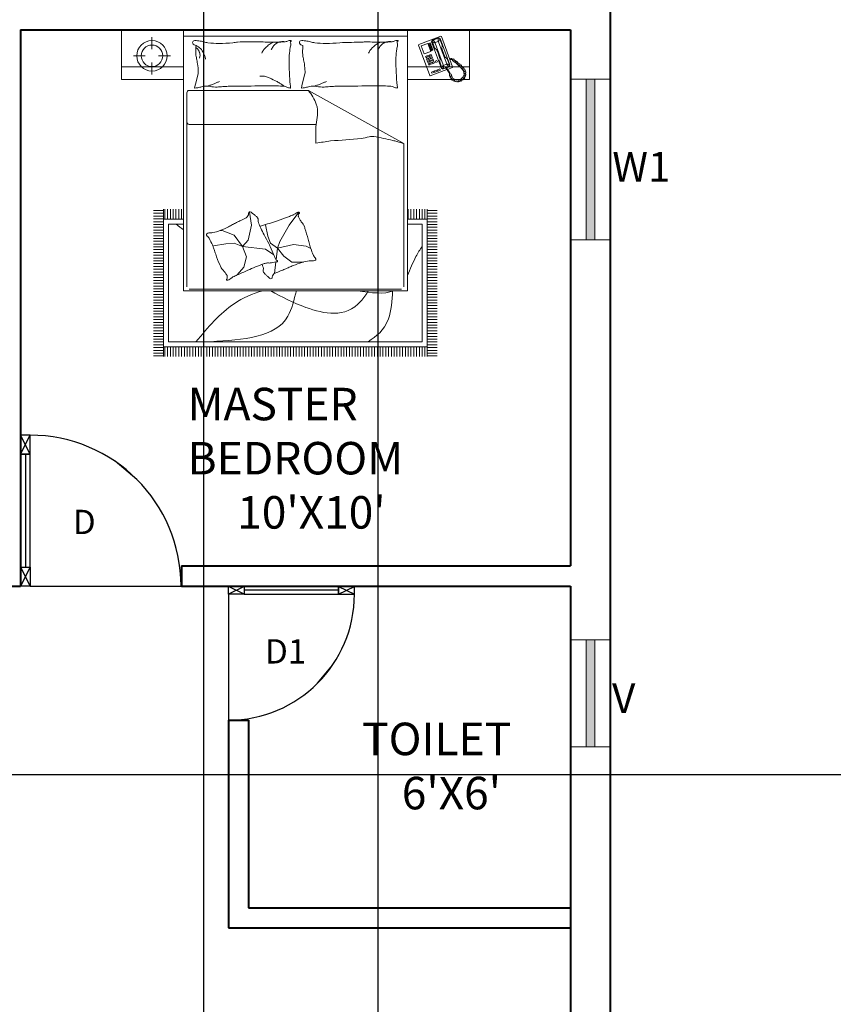
# Model space of a CAD drawing. Units: inches. Extents: x 182 to 1022, y -617 to 111.
# Tile 17 of 33: x 433 to 615, y -340 to -120. Entities that reach past the tile are written whole.
import ezdxf

# ---------------------------------------------------------------- set-up
doc = ezdxf.new("R2010")
doc.units = ezdxf.units.IN
doc.header["$MEASUREMENT"] = 0
for name, color, linetype, lineweight in [('A-ANNO-DIMS', 2, 'Continuous', 18), ('A-ANNO-IDEN', 1, 'Continuous', 18), ('A-AREA-IDEN', 8, 'Continuous', 18), ('A-GLAZ-PATT', 5, 'Continuous', 13), ('door', 2, 'Continuous', 25), ('wall', 1, 'Continuous', 40), ('wind', 5, 'Continuous', 20)]:
    doc.layers.add(name, color=color, linetype=linetype, lineweight=lineweight)
doc.layers.add('furniture', color=50, linetype='Continuous', lineweight=15, transparency=0.8)
doc.styles.add('DIM_FONT', font='SIMPLEX.shx', dxfattribs={"width": 0.8})
doc.styles.get("Standard").update_dxf_attribs({"font": 'arial.ttf'})
doc.dimstyles.get("Standard").update_dxf_attribs({"dimtxt": 0.18, "dimasz": 0.18, "dimexe": 0.18, "dimexo": 0.0625, "dimgap": 0.09, "dimtad": 0, "dimtih": 1, "dimtoh": 1, "dimdec": 1, "dimzin": 0, "dimdsep": 46, "dimlunit": 4, "dimtxsty": 'Standard', "dimcen": 0.09, "dimadec": 0, "dimazin": 0, "dimtfac": 1, "dimtdec": 1, "dimtofl": 0, "dimtmove": 0, "dimatfit": 3, "dimfxl": 1, "dimtolj": 1, "dimtzin": 0, "dimarcsym": 0})

# ---------------------------------------------------------------- blocks, each defined once
blk = doc.blocks.new('A$C2D7661C6')
for p, q in [((0, 700), (50, 800)), ((50, 700), (0, 800)), ((25, 700), (25, 100)), ((50, 100), (0, 0)), ((0, 100), (50, 0))]:
    blk.add_line(p, q)
for points in [[(0, 700), (50, 700), (50, 800), (0, 800)], [(0, 100), (50, 100), (50, 700), (0, 700)], [(0, 100), (50, 100), (50, 0), (0, 0)]]:
    blk.add_lwpolyline(points, close=True)
blk.add_arc((50, 0), 800, 0, 90)
blk = doc.blocks.new('A$C7F556C88')
for p, q in [((615.7, 565.7), (500.3, 661.3)), ((50, 0), (850, 0))]:
    blk.add_line(p, q)
blk.add_blockref('A$C2D7661C6', (0, 0))
blk = doc.blocks.new('A$C4F634EDD')
for p, q in [((0, 2.6295), (0, 2.2295)), ((0.5, 2.6295), (0, 2.6295)), ((0.5, 2.6295), (2.3, 2.6295)), ((0.5, 0.5295), (0.5, 2.6295)), ((0.5, 2.2295), (0.5, 2.6295)), ((2.3, 2.6295), (2.3, 0.5295)), ((2.3, 2.6295), (2.8, 2.6295)), ((2.3, 2.2295), (2.3, 2.6295)), ((2.8, 2.6295), (2.8, 2.2295)), ((0.2457, 2.5697), (0.2457, 2.4733)), ((0.5, 2.5771), (2.3, 2.5771)), ((2.392, 2.5115), (2.5692, 2.5765)), ((2.4946, 2.5331), (2.4985, 2.5445)), ((2.4985, 2.5445), (2.5516, 2.564)), ((2.5062, 2.5454), (2.5004, 2.5392)), ((2.5004, 2.5392), (2.5013, 2.5315)), ((2.5062, 2.5454), (2.5487, 2.561)), ((2.5235, 2.5256), (2.5062, 2.5454)), ((2.5483, 2.5347), (2.5235, 2.5256)), ((2.5483, 2.5347), (2.5487, 2.561)), ((2.5514, 2.5318), (2.5483, 2.5347)), ((2.5487, 2.561), (2.5571, 2.56)), ((2.5615, 2.5536), (2.5514, 2.5318)), ((2.5516, 2.564), (2.5637, 2.5584)), ((2.5571, 2.56), (2.5615, 2.5536)), ((2.5615, 2.5536), (2.5791, 2.5058)), ((2.5637, 2.5584), (2.6418, 2.3458)), ((2.5692, 2.5765), (2.574, 2.5743)), ((2.574, 2.5743), (2.6638, 2.3298)), ((2.3898, 2.5066), (2.392, 2.5115)), ((2.4795, 2.2621), (2.3898, 2.5066)), ((2.412, 2.5007), (2.4634, 2.5196)), ((2.4361, 2.4352), (2.412, 2.5007)), ((2.4634, 2.5196), (2.4875, 2.454)), ((2.4842, 2.5232), (2.47, 2.518)), ((2.47, 2.518), (2.472, 2.5127)), ((2.472, 2.5127), (2.4862, 2.5179)), ((2.4881, 2.5126), (2.4739, 2.5074)), ((2.4739, 2.5074), (2.4759, 2.502)), ((2.4759, 2.502), (2.4901, 2.5073)), ((2.492, 2.5019), (2.4778, 2.4967)), ((2.4778, 2.4967), (2.4798, 2.4914)), ((2.4798, 2.4914), (2.494, 2.4966)), ((2.4959, 2.4913), (2.4817, 2.4861)), ((2.4817, 2.4861), (2.4837, 2.4808)), ((2.4837, 2.4808), (2.4979, 2.486)), ((2.4862, 2.5179), (2.4842, 2.5232)), ((2.4998, 2.4807), (2.4856, 2.4755)), ((2.4856, 2.4755), (2.4876, 2.4702)), ((2.4876, 2.4702), (2.5018, 2.4754)), ((2.4901, 2.5073), (2.4881, 2.5126)), ((2.5037, 2.47), (2.4895, 2.4648)), ((2.4895, 2.4648), (2.4915, 2.4595)), ((2.4915, 2.4595), (2.5057, 2.4647)), ((2.494, 2.4966), (2.492, 2.5019)), ((2.5734, 2.3187), (2.4946, 2.5331)), ((2.4979, 2.486), (2.4959, 2.4913)), ((2.5018, 2.4754), (2.4998, 2.4807)), ((2.5013, 2.5315), (2.5188, 2.4836)), ((2.5013, 2.5315), (2.5231, 2.5214)), ((2.5057, 2.4647), (2.5037, 2.47)), ((2.5188, 2.4836), (2.5256, 2.4761)), ((2.5231, 2.5214), (2.5235, 2.5256)), ((2.5523, 2.4417), (2.5231, 2.5214)), ((2.5256, 2.4761), (2.5342, 2.4692)), ((2.5342, 2.4692), (2.5405, 2.4574)), ((2.5405, 2.4574), (2.547, 2.4397)), ((2.5807, 2.4521), (2.5514, 2.5318)), ((2.5788, 2.4956), (2.5767, 2.4848)), ((2.5767, 2.4848), (2.5795, 2.4717)), ((2.5791, 2.5058), (2.5788, 2.4956)), ((2.5795, 2.4717), (2.586, 2.454)), ((0.0957, 2.4197), (0.192, 2.4197)), ((0.2994, 2.4197), (0.3957, 2.4197)), ((2.4875, 2.454), (2.4361, 2.4352)), ((2.4457, 2.4146), (2.4563, 2.4185)), ((2.4496, 2.4039), (2.4457, 2.4146)), ((2.4602, 2.4078), (2.4496, 2.4039)), ((2.4528, 2.3951), (2.4635, 2.399)), ((2.4567, 2.3844), (2.4528, 2.3951)), ((2.4563, 2.4185), (2.4602, 2.4078)), ((2.4674, 2.3883), (2.4567, 2.3844)), ((2.46, 2.3756), (2.4706, 2.3795)), ((2.4634, 2.4211), (2.474, 2.425)), ((2.4673, 2.4104), (2.4634, 2.4211)), ((2.4635, 2.399), (2.4674, 2.3883)), ((2.4779, 2.4143), (2.4673, 2.4104)), ((2.4706, 2.4016), (2.4812, 2.4055)), ((2.4745, 2.3909), (2.4706, 2.4016)), ((2.4706, 2.3795), (2.4745, 2.3689)), ((2.474, 2.425), (2.4779, 2.4143)), ((2.4851, 2.3949), (2.4745, 2.3909)), ((2.4777, 2.3821), (2.4883, 2.386)), ((2.4816, 2.3715), (2.4777, 2.3821)), ((2.4811, 2.4276), (2.4917, 2.4315)), ((2.485, 2.4169), (2.4811, 2.4276)), ((2.4812, 2.4055), (2.4851, 2.3949)), ((2.4956, 2.4208), (2.485, 2.4169)), ((2.4883, 2.4081), (2.4989, 2.412)), ((2.4922, 2.3975), (2.4883, 2.4081)), ((2.4883, 2.386), (2.4922, 2.3754)), ((2.4917, 2.4315), (2.4956, 2.4208)), ((2.5028, 2.4014), (2.4922, 2.3975)), ((2.4954, 2.3886), (2.5061, 2.3925)), ((2.4993, 2.378), (2.4954, 2.3886)), ((2.4989, 2.412), (2.5028, 2.4014)), ((2.51, 2.3819), (2.4993, 2.378)), ((2.5061, 2.3925), (2.51, 2.3819)), ((2.5238, 2.3769), (2.538, 2.3821)), ((2.5277, 2.3663), (2.5238, 2.3769)), ((2.538, 2.3821), (2.5419, 2.3715)), ((2.5594, 2.4061), (2.547, 2.4397)), ((2.5523, 2.4417), (2.5875, 2.346)), ((2.5622, 2.393), (2.5594, 2.4061)), ((2.5598, 2.372), (2.5601, 2.3822)), ((2.5601, 2.3822), (2.5622, 2.393)), ((2.5807, 2.4521), (2.6158, 2.3564)), ((2.5984, 2.4204), (2.586, 2.454)), ((2.6047, 2.4086), (2.5984, 2.4204)), ((2.6133, 2.4017), (2.6047, 2.4086)), ((2.6201, 2.3941), (2.6133, 2.4017)), ((2.6376, 2.3463), (2.6201, 2.3941)), ((2.6499, 2.3979), (2.6397, 2.3953)), ((2.6417, 2.39), (2.6488, 2.391)), ((2.6488, 2.391), (2.6538, 2.3895)), ((2.6551, 2.397), (2.6499, 2.3979)), ((2.6538, 2.3895), (2.6596, 2.388)), ((2.6627, 2.392), (2.6551, 2.397)), ((2.6596, 2.388), (2.6626, 2.3867)), ((2.6626, 2.3867), (2.6662, 2.388)), ((2.6692, 2.394), (2.6627, 2.392)), ((2.6662, 2.388), (2.6632, 2.3828)), ((2.6632, 2.3828), (2.6736, 2.3744)), ((2.6736, 2.3944), (2.6692, 2.394)), ((2.6765, 2.391), (2.6736, 2.3944)), ((2.6742, 2.3795), (2.6765, 2.391)), ((2.6824, 2.3858), (2.6742, 2.3795)), ((2.6873, 2.3815), (2.6824, 2.3858)), ((2.6853, 2.369), (2.6873, 2.3815)), ((0, 2.3301), (0.5, 2.3301)), ((0.2457, 2.366), (0.2457, 2.2697)), ((2.8, 2.3301), (2.3, 2.3301)), ((2.4639, 2.365), (2.46, 2.3756)), ((2.4745, 2.3689), (2.4639, 2.365)), ((2.4672, 2.3561), (2.4778, 2.36)), ((2.4711, 2.3455), (2.4672, 2.3561)), ((2.4817, 2.3494), (2.4711, 2.3455)), ((2.4778, 2.36), (2.4817, 2.3494)), ((2.4922, 2.3754), (2.4816, 2.3715)), ((2.6172, 2.3086), (2.4844, 2.2599)), ((2.4849, 2.3626), (2.4955, 2.3665)), ((2.4888, 2.352), (2.4849, 2.3626)), ((2.4994, 2.3559), (2.4888, 2.352)), ((2.4955, 2.3665), (2.4994, 2.3559)), ((2.5026, 2.3691), (2.5132, 2.373)), ((2.5065, 2.3585), (2.5026, 2.3691)), ((2.5171, 2.3624), (2.5065, 2.3585)), ((2.5132, 2.373), (2.5171, 2.3624)), ((2.5362, 2.305), (2.5185, 2.2985)), ((2.5185, 2.2985), (2.5224, 2.2879)), ((2.5419, 2.3715), (2.5277, 2.3663)), ((2.5401, 2.2944), (2.5362, 2.305)), ((2.561, 2.3141), (2.5433, 2.3076)), ((2.5433, 2.3076), (2.5472, 2.297)), ((2.5472, 2.297), (2.5649, 2.3035)), ((2.5774, 2.3242), (2.5598, 2.372)), ((2.5649, 2.3035), (2.561, 2.3141)), ((2.5855, 2.3131), (2.5734, 2.3187)), ((2.5774, 2.3242), (2.5875, 2.346)), ((2.5818, 2.3178), (2.5774, 2.3242)), ((2.5901, 2.3168), (2.5818, 2.3178)), ((2.6104, 2.3222), (2.5855, 2.3131)), ((2.5875, 2.346), (2.5905, 2.3431)), ((2.5905, 2.3431), (2.5901, 2.3168)), ((2.5901, 2.3168), (2.6097, 2.324)), ((2.6154, 2.3522), (2.5905, 2.3431)), ((2.613, 2.3312), (2.6077, 2.3293)), ((2.6077, 2.3293), (2.6135, 2.3141)), ((2.6192, 2.3174), (2.613, 2.3312)), ((2.6135, 2.3141), (2.6244, 2.2977)), ((2.6153, 2.3261), (2.6327, 2.3324)), ((2.6158, 2.3564), (2.6154, 2.3522)), ((2.6154, 2.3522), (2.6327, 2.3324)), ((2.6376, 2.3463), (2.6158, 2.3564)), ((2.6369, 2.332), (2.6161, 2.3243)), ((2.626, 2.3069), (2.6192, 2.3174)), ((2.6616, 2.3249), (2.6234, 2.3109)), ((2.6244, 2.2977), (2.6349, 2.2825)), ((2.6365, 2.2916), (2.626, 2.3069)), ((2.6327, 2.3324), (2.6385, 2.3386)), ((2.6418, 2.3458), (2.6369, 2.332)), ((2.6385, 2.3386), (2.6376, 2.3463)), ((2.6638, 2.3298), (2.6616, 2.3249)), ((2.6736, 2.3744), (2.6922, 2.3593)), ((2.6946, 2.376), (2.6853, 2.369)), ((2.6922, 2.3593), (2.7051, 2.3473)), ((2.6995, 2.3713), (2.6946, 2.376)), ((2.695, 2.3603), (2.6995, 2.3713)), ((2.7031, 2.3682), (2.695, 2.3603)), ((2.7096, 2.3616), (2.7031, 2.3682)), ((2.7051, 2.3473), (2.7079, 2.3475)), ((2.7062, 2.351), (2.7096, 2.3616)), ((2.7147, 2.3578), (2.7062, 2.351)), ((2.7079, 2.3475), (2.7079, 2.3443)), ((2.7079, 2.3443), (2.727, 2.3277)), ((2.7214, 2.3517), (2.7147, 2.3578)), ((2.7196, 2.34), (2.7214, 2.3517)), ((2.7286, 2.3466), (2.7196, 2.34)), ((2.727, 2.3277), (2.7512, 2.2983)), ((2.7346, 2.3423), (2.7286, 2.3466)), ((2.732, 2.3295), (2.7346, 2.3423)), ((2.7423, 2.3345), (2.732, 2.3295)), ((2.7406, 2.3172), (2.7495, 2.325)), ((2.7519, 2.3218), (2.7406, 2.3172)), ((2.7495, 2.325), (2.7423, 2.3345)), ((2.7512, 2.2983), (2.756, 2.2695)), ((2.7575, 2.3144), (2.7519, 2.3218)), ((2.7526, 2.3045), (2.7575, 2.3144)), ((2.7622, 2.308), (2.7526, 2.3045)), ((2.7574, 2.2924), (2.7673, 2.2997)), ((2.7673, 2.2997), (2.7622, 2.308)), ((0, 2.2295), (0.5, 2.2295)), ((0.5953, 2.1912), (0.616, 2.2738)), ((1.4546, 2.1912), (1.4752, 2.2738)), ((2.8, 2.2295), (2.3, 2.2295)), ((2.4844, 2.2599), (2.4795, 2.2621)), ((2.5114, 2.2959), (2.4936, 2.2894)), ((2.4936, 2.2894), (2.4976, 2.2788)), ((2.4976, 2.2788), (2.5153, 2.2853)), ((2.5153, 2.2853), (2.5114, 2.2959)), ((2.5224, 2.2879), (2.5401, 2.2944)), ((2.6349, 2.2825), (2.638, 2.273)), ((2.6407, 2.2834), (2.6365, 2.2916)), ((2.6399, 2.2712), (2.6374, 2.2659)), ((2.6374, 2.2659), (2.6398, 2.257)), ((2.638, 2.273), (2.6399, 2.2712)), ((2.6398, 2.257), (2.6509, 2.259)), ((2.6438, 2.2739), (2.6407, 2.2834)), ((2.6509, 2.259), (2.6431, 2.2492)), ((2.6431, 2.2492), (2.6473, 2.2398)), ((2.6519, 2.2716), (2.6438, 2.2739)), ((2.6473, 2.2398), (2.6592, 2.2429)), ((2.6535, 2.2628), (2.6519, 2.2716)), ((2.6592, 2.2429), (2.6521, 2.2314)), ((2.6521, 2.2314), (2.6598, 2.2248)), ((2.6636, 2.2409), (2.6535, 2.2628)), ((2.6598, 2.2248), (2.6697, 2.2309)), ((2.6836, 2.2287), (2.6636, 2.2409)), ((2.6697, 2.2309), (2.6684, 2.219)), ((2.6684, 2.219), (2.6761, 2.2145)), ((2.6761, 2.2145), (2.6821, 2.2237)), ((2.6821, 2.2237), (2.6843, 2.2135)), ((2.7063, 2.2256), (2.6836, 2.2287)), ((2.6927, 2.2117), (2.6986, 2.222)), ((2.6986, 2.222), (2.7019, 2.2098)), ((2.7284, 2.2317), (2.7063, 2.2256)), ((2.7102, 2.2104), (2.7113, 2.2218)), ((2.7113, 2.2218), (2.7192, 2.2137)), ((2.7255, 2.2152), (2.7242, 2.2265)), ((2.7242, 2.2265), (2.7324, 2.2165)), ((2.7459, 2.2483), (2.7284, 2.2317)), ((2.7324, 2.2165), (2.7386, 2.2208)), ((2.7386, 2.2208), (2.7354, 2.2306)), ((2.7354, 2.2306), (2.7462, 2.2264)), ((2.756, 2.2695), (2.7459, 2.2483)), ((2.7509, 2.2314), (2.7459, 2.2418)), ((2.7459, 2.2418), (2.7568, 2.2352)), ((2.7462, 2.2264), (2.7509, 2.2314)), ((2.7529, 2.2505), (2.7645, 2.2498)), ((2.7607, 2.2424), (2.7529, 2.2505)), ((2.7568, 2.2352), (2.7607, 2.2424)), ((2.7687, 2.2905), (2.7574, 2.2924)), ((2.7587, 2.279), (2.7699, 2.2828)), ((2.7708, 2.2725), (2.7587, 2.279)), ((2.759, 2.2637), (2.7706, 2.2643)), ((2.7676, 2.2559), (2.759, 2.2637)), ((2.7645, 2.2498), (2.7676, 2.2559)), ((2.7699, 2.2828), (2.7687, 2.2905)), ((2.7706, 2.2643), (2.7708, 2.2725)), ((1.5035, 2.141), (0.5458, 2.141)), ((0.5878, 2.1612), (0.5953, 2.1912)), ((1.4471, 2.1612), (1.4546, 2.1912)), ((1.5035, 2.141), (2.2716, 1.7136)), ((2.6843, 2.2135), (2.6927, 2.2117)), ((2.7019, 2.2098), (2.7102, 2.2104)), ((2.7192, 2.2137), (2.7255, 2.2152)), ((0.5258, 2.121), (0.5258, 0.5617)), ((1.576, 1.9433), (1.5624, 1.8479)), ((0.5458, 1.8684), (1.5653, 1.8684)), ((1.5624, 1.8479), (1.5641, 1.7178)), ((2.2716, 0.5617), (2.2716, 1.7136)), ((0.2586, 1.1753), (0.3386, 1.1753)), ((0.2586, 1.1528), (0.3386, 1.1528)), ((0.2586, 1.1303), (0.3386, 1.1303)), ((0.3386, 0), (0.3386, 1.1852)), ((0.3486, 1.1052), (0.3486, 1.1852)), ((0.3711, 1.1052), (0.3711, 1.1852)), ((0.3936, 1.1052), (0.3936, 1.1852)), ((0.4161, 1.1052), (0.4161, 1.1852)), ((0.4386, 1.1052), (0.4386, 1.1852)), ((0.4611, 1.1052), (0.4611, 1.1852)), ((0.4836, 1.1052), (0.4836, 1.1852)), ((1.031, 1.1612), (1.0448, 1.0581)), ((1.4276, 1.1611), (1.3484, 1.0571)), ((2.3061, 1.1052), (2.3061, 1.1852)), ((2.3286, 1.1052), (2.3286, 1.1852)), ((2.3511, 1.1052), (2.3511, 1.1852)), ((2.3736, 1.1052), (2.3736, 1.1852)), ((2.3961, 1.1052), (2.3961, 1.1852)), ((2.4186, 1.1052), (2.4186, 1.1852)), ((2.4411, 1.1052), (2.4411, 1.1852)), ((2.4588, 1.1852), (2.4588, 0)), ((2.4588, 1.1753), (2.5388, 1.1753)), ((2.4588, 1.1528), (2.5388, 1.1528)), ((2.4588, 1.1303), (2.5388, 1.1303)), ((0.2586, 1.1078), (0.3386, 1.1078)), ((0.2586, 1.0853), (0.3386, 1.0853)), ((0.2586, 1.0628), (0.3386, 1.0628)), ((0.2586, 1.0403), (0.3386, 1.0403)), ((0.3386, 1.1052), (0.5, 1.1052)), ((0.3786, 1.0652), (0.5, 1.0652)), ((0.3786, 0.12), (0.3786, 1.0652)), ((1.0448, 1.0581), (1.019, 0.936)), ((1.1784, 0.9702), (1.1586, 1.0591)), ((1.3484, 1.0571), (1.2733, 0.9268)), ((2.3, 1.1052), (2.4588, 1.1052)), ((2.3, 1.0652), (2.4188, 1.0652)), ((2.4188, 1.0652), (2.4188, 0.12)), ((2.4588, 1.1078), (2.5388, 1.1078)), ((2.4588, 1.0853), (2.5388, 1.0853)), ((2.4588, 1.0628), (2.5388, 1.0628)), ((2.4588, 1.0403), (2.5388, 1.0403)), ((0.2586, 1.0178), (0.3386, 1.0178)), ((0.2586, 0.9953), (0.3386, 0.9953)), ((0.2586, 0.9728), (0.3386, 0.9728)), ((0.8108, 1.0151), (0.7868, 1.0117)), ((0.9054, 0.9773), (0.8108, 1.0151)), ((0.9743, 0.8845), (0.9054, 0.9773)), ((1.1982, 0.9129), (1.1784, 0.9702)), ((2.4588, 1.0178), (2.5388, 1.0178)), ((2.4588, 0.9953), (2.5388, 0.9953)), ((2.4588, 0.9728), (2.5388, 0.9728)), ((0.2586, 0.9503), (0.3386, 0.9503)), ((0.2586, 0.9278), (0.3386, 0.9278)), ((0.2586, 0.9053), (0.3386, 0.9053)), ((0.2586, 0.8828), (0.3386, 0.8828)), ((0.7403, 0.8913), (0.737, 0.8849)), ((0.8384, 0.9085), (0.7403, 0.8913)), ((0.9072, 0.912), (0.8384, 0.9085)), ((0.9743, 0.8845), (0.9072, 0.912)), ((1.019, 0.936), (0.9743, 0.8845)), ((0.9743, 0.8845), (1.0052, 0.802)), ((0.9743, 0.8845), (1.16, 0.8656)), ((1.1973, 0.8853), (1.2203, 0.829)), ((1.2555, 0.8715), (1.1982, 0.9129)), ((1.2555, 0.8715), (1.2437, 0.7773)), ((1.2733, 0.9268), (1.2555, 0.8715)), ((1.2555, 0.8715), (1.384, 0.9031)), ((1.2555, 0.8715), (1.3049, 0.8082)), ((1.384, 0.9031), (1.4868, 0.8892)), ((1.4868, 0.8892), (1.5228, 0.8692)), ((2.4588, 0.9503), (2.5388, 0.9503)), ((2.4588, 0.9278), (2.5388, 0.9278)), ((2.4588, 0.9053), (2.5388, 0.9053)), ((2.4588, 0.8828), (2.5388, 0.8828)), ((0.2586, 0.8603), (0.3386, 0.8603)), ((0.2586, 0.8378), (0.3386, 0.8378)), ((0.2586, 0.8153), (0.3386, 0.8153)), ((0.2586, 0.7928), (0.3386, 0.7928)), ((1.0052, 0.802), (0.9846, 0.7194)), ((1.16, 0.8656), (1.2099, 0.8295)), ((1.2099, 0.8295), (1.222, 0.8209)), ((1.2203, 0.829), (1.2381, 0.7855)), ((1.3049, 0.8082), (1.3701, 0.7608)), ((2.4588, 0.8603), (2.5388, 0.8603)), ((2.4588, 0.8378), (2.5388, 0.8378)), ((2.4588, 0.8153), (2.5388, 0.8153)), ((2.4588, 0.7928), (2.5388, 0.7928)), ((0.2586, 0.7703), (0.3386, 0.7703)), ((0.2586, 0.7478), (0.3386, 0.7478)), ((0.2586, 0.7253), (0.3386, 0.7253)), ((0.9846, 0.7194), (0.931, 0.6569)), ((1.2419, 0.7626), (1.23, 0.668)), ((1.3701, 0.7608), (1.463, 0.7608)), ((2.4588, 0.7703), (2.5388, 0.7703)), ((2.4588, 0.7478), (2.5388, 0.7478)), ((2.4588, 0.7253), (2.5388, 0.7253)), ((0.2586, 0.7028), (0.3386, 0.7028)), ((0.2586, 0.6803), (0.3386, 0.6803)), ((0.2586, 0.6578), (0.3386, 0.6578)), ((0.2586, 0.6353), (0.3386, 0.6353)), ((2.4588, 0.7028), (2.5388, 0.7028)), ((2.4588, 0.6803), (2.5388, 0.6803)), ((2.4588, 0.6578), (2.5388, 0.6578)), ((2.4588, 0.6353), (2.5388, 0.6353)), ((0.2586, 0.6128), (0.3386, 0.6128)), ((0.2586, 0.5903), (0.3386, 0.5903)), ((0.2586, 0.5678), (0.3386, 0.5678)), ((2.4588, 0.6128), (2.5388, 0.6128)), ((2.4588, 0.5903), (2.5388, 0.5903)), ((2.4588, 0.5678), (2.5388, 0.5678)), ((0.2586, 0.5453), (0.3386, 0.5453)), ((0.2586, 0.5228), (0.3386, 0.5228)), ((0.2586, 0.5003), (0.3386, 0.5003)), ((0.2586, 0.4778), (0.3386, 0.4778)), ((2.3, 0.5295), (0.5, 0.5295)), ((0.5458, 0.5417), (2.2516, 0.5417)), ((2.4588, 0.5453), (2.5388, 0.5453)), ((2.4588, 0.5228), (2.5388, 0.5228)), ((2.4588, 0.5003), (2.5388, 0.5003)), ((2.4588, 0.4778), (2.5388, 0.4778)), ((0.2586, 0.4553), (0.3386, 0.4553)), ((0.2586, 0.4328), (0.3386, 0.4328)), ((0.2586, 0.4103), (0.3386, 0.4103)), ((2.4588, 0.4553), (2.5388, 0.4553)), ((2.4588, 0.4328), (2.5388, 0.4328)), ((2.4588, 0.4103), (2.5388, 0.4103)), ((0.2586, 0.3878), (0.3386, 0.3878)), ((0.2586, 0.3653), (0.3386, 0.3653)), ((0.2586, 0.3428), (0.3386, 0.3428)), ((0.2586, 0.3203), (0.3386, 0.3203)), ((2.4588, 0.3878), (2.5388, 0.3878)), ((2.4588, 0.3653), (2.5388, 0.3653)), ((2.4588, 0.3428), (2.5388, 0.3428)), ((2.4588, 0.3203), (2.5388, 0.3203)), ((0.2586, 0.2978), (0.3386, 0.2978)), ((0.2586, 0.2753), (0.3386, 0.2753)), ((0.2586, 0.2528), (0.3386, 0.2528)), ((2.4588, 0.2978), (2.5388, 0.2978)), ((2.4588, 0.2753), (2.5388, 0.2753)), ((2.4588, 0.2528), (2.5388, 0.2528)), ((0.2586, 0.2303), (0.3386, 0.2303)), ((0.2586, 0.2078), (0.3386, 0.2078)), ((0.2586, 0.1853), (0.3386, 0.1853)), ((0.2586, 0.1628), (0.3386, 0.1628)), ((2.4588, 0.2303), (2.5388, 0.2303)), ((2.4588, 0.2078), (2.5388, 0.2078)), ((2.4588, 0.1853), (2.5388, 0.1853)), ((2.4588, 0.1628), (2.5388, 0.1628)), ((0.2586, 0.1403), (0.3386, 0.1403)), ((0.2586, 0.1178), (0.3386, 0.1178)), ((0.2586, 0.0953), (0.3386, 0.0953)), ((2.4588, 0.08), (0.3386, 0.08)), ((0.3486, 0), (0.3486, 0.08)), ((0.3711, 0), (0.3711, 0.08)), ((2.4188, 0.12), (0.3786, 0.12)), ((0.3936, 0), (0.3936, 0.08)), ((0.4161, 0), (0.4161, 0.08)), ((0.4386, 0), (0.4386, 0.08)), ((0.4611, 0), (0.4611, 0.08)), ((0.4836, 0), (0.4836, 0.08)), ((0.5061, 0), (0.5061, 0.08)), ((0.5286, 0), (0.5286, 0.08)), ((0.5511, 0), (0.5511, 0.08)), ((0.5736, 0), (0.5736, 0.08)), ((0.5961, 0), (0.5961, 0.08)), ((0.6186, 0), (0.6186, 0.08)), ((0.6411, 0), (0.6411, 0.08)), ((0.6636, 0), (0.6636, 0.08)), ((0.6861, 0), (0.6861, 0.08)), ((0.7086, 0), (0.7086, 0.08)), ((0.7311, 0), (0.7311, 0.08)), ((0.7536, 0), (0.7536, 0.08)), ((0.7761, 0), (0.7761, 0.08)), ((0.7986, 0), (0.7986, 0.08)), ((0.8211, 0), (0.8211, 0.08)), ((0.8436, 0), (0.8436, 0.08)), ((0.8661, 0), (0.8661, 0.08)), ((0.8886, 0), (0.8886, 0.08)), ((0.9111, 0), (0.9111, 0.08)), ((0.9336, 0), (0.9336, 0.08)), ((0.9561, 0), (0.9561, 0.08)), ((0.9786, 0), (0.9786, 0.08)), ((1.0011, 0), (1.0011, 0.08)), ((1.0236, 0), (1.0236, 0.08)), ((1.0461, 0), (1.0461, 0.08)), ((1.0686, 0), (1.0686, 0.08)), ((1.0911, 0), (1.0911, 0.08)), ((1.1136, 0), (1.1136, 0.08)), ((1.1361, 0), (1.1361, 0.08)), ((1.1586, 0), (1.1586, 0.08)), ((1.1811, 0), (1.1811, 0.08)), ((1.2036, 0), (1.2036, 0.08)), ((1.2261, 0), (1.2261, 0.08)), ((1.2486, 0), (1.2486, 0.08)), ((1.2711, 0), (1.2711, 0.08)), ((1.2936, 0), (1.2936, 0.08)), ((1.3161, 0), (1.3161, 0.08)), ((1.3386, 0), (1.3386, 0.08)), ((1.3611, 0), (1.3611, 0.08)), ((1.3836, 0), (1.3836, 0.08)), ((1.4061, 0), (1.4061, 0.08)), ((1.4286, 0), (1.4286, 0.08)), ((1.4511, 0), (1.4511, 0.08)), ((1.4736, 0), (1.4736, 0.08)), ((1.4961, 0), (1.4961, 0.08)), ((1.5186, 0), (1.5186, 0.08)), ((1.5411, 0), (1.5411, 0.08)), ((1.5636, 0), (1.5636, 0.08)), ((1.5861, 0), (1.5861, 0.08)), ((1.6086, 0), (1.6086, 0.08)), ((1.6311, 0), (1.6311, 0.08)), ((1.6536, 0), (1.6536, 0.08)), ((1.6761, 0), (1.6761, 0.08)), ((1.6986, 0), (1.6986, 0.08)), ((1.7211, 0), (1.7211, 0.08)), ((1.7436, 0), (1.7436, 0.08)), ((1.7661, 0), (1.7661, 0.08)), ((1.7886, 0), (1.7886, 0.08)), ((1.8111, 0), (1.8111, 0.08)), ((1.8336, 0), (1.8336, 0.08)), ((1.8561, 0), (1.8561, 0.08)), ((1.8786, 0), (1.8786, 0.08)), ((1.9011, 0), (1.9011, 0.08)), ((1.9236, 0), (1.9236, 0.08)), ((1.9461, 0), (1.9461, 0.08)), ((1.9686, 0), (1.9686, 0.08)), ((1.9911, 0), (1.9911, 0.08)), ((2.0136, 0), (2.0136, 0.08)), ((2.0361, 0), (2.0361, 0.08)), ((2.0586, 0), (2.0586, 0.08)), ((2.0811, 0), (2.0811, 0.08)), ((2.1036, 0), (2.1036, 0.08)), ((2.1261, 0), (2.1261, 0.08)), ((2.1486, 0), (2.1486, 0.08)), ((2.1711, 0), (2.1711, 0.08)), ((2.1936, 0), (2.1936, 0.08)), ((2.2161, 0), (2.2161, 0.08)), ((2.2386, 0), (2.2386, 0.08)), ((2.2611, 0), (2.2611, 0.08)), ((2.2836, 0), (2.2836, 0.08)), ((2.3061, 0), (2.3061, 0.08)), ((2.3286, 0), (2.3286, 0.08)), ((2.3511, 0), (2.3511, 0.08)), ((2.3736, 0), (2.3736, 0.08)), ((2.3961, 0), (2.3961, 0.08)), ((2.4186, 0), (2.4186, 0.08)), ((2.4411, 0), (2.4411, 0.08)), ((2.4588, 0.1403), (2.5388, 0.1403)), ((2.4588, 0.1178), (2.5388, 0.1178)), ((2.4588, 0.0953), (2.5388, 0.0953)), ((0.2586, 0.0728), (0.3386, 0.0728)), ((0.2586, 0.0503), (0.3386, 0.0503)), ((0.2586, 0.0278), (0.3386, 0.0278)), ((0.2586, 0.0053), (0.3386, 0.0053)), ((2.4588, 0.0728), (2.5388, 0.0728)), ((2.4588, 0.0503), (2.5388, 0.0503)), ((2.4588, 0.0278), (2.5388, 0.0278)), ((2.4588, 0.0053), (2.5388, 0.0053))]:
    blk.add_line(p, q)
for radius in [0.1222, 0.0865]:
    blk.add_circle((0.2457, 2.4197), radius)
for centre, radius, start, end in [((0.5848, 2.5274), 0.0131, 101.27238, 206.58052), ((0.5999, 2.4516), 0.0904, 90, 101.27238), ((0.5999, 2.3808), 0.1611, 81.56281, 90), ((0.5788, 2.2388), 0.3048, 74.25602, 81.56281), ((1.2995, 2.4357), 0.0992, 85.78412, 105.93524), ((1.3132, 2.5864), 0.0539, 275.25919, 300.65125), ((1.3554, 2.5152), 0.0289, 85.69746, 120.65125), ((1.3556, 2.519), 0.0251, 68.2117, 85.69746), ((1.3739, 2.5288), 0.0156, 158.0096, 201.42098), ((1.3634, 2.533), 0.00428, 78.10694, 158.0096), ((1.3647, 2.5395), 0.00232, 258.10694, 19.56397), ((1.3637, 2.5391), 0.00342, 19.56397, 68.2117), ((1.444, 2.5274), 0.0131, 101.27238, 206.58052), ((1.4591, 2.4516), 0.0904, 90, 101.27238), ((1.4591, 2.3808), 0.1611, 81.56281, 90), ((1.438, 2.2388), 0.3048, 74.25602, 81.56281), ((2.1588, 2.4357), 0.0992, 85.78412, 105.93524), ((2.1724, 2.5864), 0.0539, 275.25919, 300.65125), ((2.2146, 2.5152), 0.0289, 85.69746, 120.65125), ((2.2149, 2.519), 0.0251, 68.2117, 85.69746), ((2.2331, 2.5288), 0.0156, 158.0096, 201.42098), ((2.2226, 2.533), 0.00428, 78.10694, 158.0096), ((2.224, 2.5395), 0.00232, 258.10694, 19.56397), ((2.2229, 2.5391), 0.00342, 19.56397, 68.2117), ((0.6036, 2.5368), 0.0342, 206.58052, 265.59979), ((1.0898, 2.4496), 0.4918, 173.76764, 180), ((0.5462, 2.4142), 0.0899, 41.44291, 53.73593), ((0.5368, 2.3783), 0.1399, 45.09762, 62.79641), ((0.5741, 2.4389), 0.0526, 25.35512, 41.44291), ((0.4851, 2.3967), 0.1511, 21.81492, 25.35512), ((0.5368, 2.3783), 0.1399, 27.39883, 45.09762), ((0.7272, 2.7653), 0.2422, 254.25602, 262.45315), ((0.7851, 3.2019), 0.6827, 262.45315, 270), ((0.7851, 3.5682), 1.049, 270, 276.0867), ((0.8402, 3.0514), 0.5293, 276.0867, 280.18988), ((1.1602, -8.1346), 10.6675, 90.30153, 91.21582), ((1.1169, 2.2433), 0.2897, 85.19815, 92.53859), ((1.3127, 2.3625), 0.2002, 151.68324, 156.99723), ((1.1799, 2.4341), 0.0493, 140.96506, 151.68324), ((1.2142, 3.4021), 0.8732, 265.19815, 269.42426), ((1.3165, 2.3233), 0.2252, 133.81151, 140.96506), ((1.4317, 2.2032), 0.3916, 128.38857, 133.81151), ((1.2362, 2.45), 0.0768, 117.23959, 128.38857), ((1.3082, 2.3102), 0.234, 110.86028, 117.23959), ((1.2204, 4.0232), 1.4943, 269.42426, 271.90789), ((1.2995, 2.4357), 0.0992, 143.82335, 161.56035), ((1.2995, 2.4357), 0.0992, 126.08636, 143.82335), ((1.2995, 2.4357), 0.0992, 105.93524, 126.08636), ((1.2429, 3.3501), 0.8208, 271.90789, 275.25919), ((2.2605, 2.3525), 0.9131, 172.3191, 176.63125), ((1.5522, 2.448), 0.1983, 167.89054, 172.3191), ((1.1177, 2.5413), 0.246, 347.89054, 351.86652), ((1.3288, 2.5111), 0.0328, 351.86652, 21.42098), ((1.4628, 2.5368), 0.0342, 206.58052, 265.59979), ((1.949, 2.4496), 0.4918, 173.76764, 180), ((1.5865, 2.7653), 0.2422, 254.25602, 262.45315), ((1.6443, 3.2019), 0.6827, 262.45315, 270), ((1.6443, 3.5682), 1.049, 270, 276.0867), ((1.4785, 15.4878), 12.9656, 271.22425, 272.05324), ((1.97, 2.3805), 0.1524, 92.53859, 100.18988), ((1.9761, 2.2433), 0.2897, 85.19815, 92.53859), ((2.1719, 2.3625), 0.2002, 151.68324, 156.99723), ((2.0391, 2.4341), 0.0493, 140.96506, 151.68324), ((2.0734, 3.4021), 0.8732, 265.19815, 269.42426), ((2.1757, 2.3233), 0.2252, 133.81151, 140.96506), ((2.291, 2.2032), 0.3916, 128.38857, 133.81151), ((2.0954, 2.45), 0.0768, 117.23959, 128.38857), ((2.1674, 2.3102), 0.234, 110.86028, 117.23959), ((2.0797, 4.0232), 1.4943, 269.42426, 271.90789), ((2.1588, 2.4357), 0.0992, 143.82335, 161.56035), ((2.1588, 2.4357), 0.0992, 126.08636, 143.82335), ((2.1588, 2.4357), 0.0992, 105.93524, 126.08636), ((2.1021, 3.3501), 0.8208, 271.90789, 275.25919), ((3.1198, 2.3525), 0.9131, 172.3191, 176.63125), ((2.4114, 2.448), 0.1983, 167.89054, 172.3191), ((1.977, 2.5413), 0.246, 347.89054, 351.86652), ((2.1881, 2.5111), 0.0328, 351.86652, 21.42098), ((0.8019, 2.4496), 0.204, 180, 189.68437), ((1.4703, 2.5637), 0.882, 189.68437, 192.19838), ((0.2982, 2.3103), 0.3171, 8.00505, 12.19838), ((0.4345, 2.3765), 0.2056, 18.7799, 21.81492), ((0.576, 2.4246), 0.0562, 0, 18.7799), ((0.5406, 2.4246), 0.0915, 345.31489, 0), ((0.5368, 2.3783), 0.1399, 16.51498, 27.39883), ((0.5368, 2.3783), 0.1399, 5.63113, 16.51498), ((2.0266, 2.3663), 0.6787, 176.63125, 181.63309), ((1.6611, 2.4496), 0.204, 180, 189.68437), ((2.3295, 2.5637), 0.882, 189.68437, 192.19838), ((1.1575, 2.3103), 0.3171, 8.00505, 12.19838), ((2.8858, 2.3663), 0.6787, 176.63125, 181.63309), ((-0.0401, 2.2627), 0.6588, 2.66488, 8.00505), ((2.7128, 2.3859), 1.3652, 181.63309, 183.05496), ((14.9657, 3.0398), 13.6356, 183.05496, 183.50486), ((0.8191, 2.2627), 0.6588, 2.66488, 8.00505), ((3.5721, 2.3859), 1.3652, 181.63309, 183.05496), ((15.8249, 3.0398), 13.6356, 183.05496, 183.50486), ((0.5503, 2.2902), 0.0677, 345.95481, 2.66488), ((1.1303, 1.9835), 0.2721, 85.91723, 93.5552), ((1.1455, 2.197), 0.058, 69.32572, 85.91723), ((0.9871, 1.7772), 0.5066, 65.67347, 69.32572), ((0.6058, 0.9338), 1.4323, 63.50152, 65.67347), ((1.4096, 2.2902), 0.0677, 345.95481, 2.66488), ((0.5458, 2.121), 0.02, 90, 180), ((0.5887, 2.1609), 0.000917, 165.95506, 274.08294), ((0.5695, 2.4301), 0.2708, 274.08294, 279.4841), ((0.5763, 2.3896), 0.2297, 279.4841, 287.38641), ((0.6807, 2.0561), 0.1197, 96.43405, 107.38641), ((0.6836, 2.0301), 0.1459, 78.44144, 96.43405), ((0.473, 2.8815), 0.7387, 287.19822, 289.42798), ((0.759, 2.3985), 0.2301, 258.44144, 272.74906), ((0.473, 2.8815), 0.7387, 289.42798, 291.65774), ((0.473, 2.8815), 0.7387, 291.65774, 293.48441), ((0.473, 2.8815), 0.7387, 293.48441, 295.31107), ((0.7026, 3.5718), 1.4048, 272.74906, 274.61758), ((0.9136, 0.9591), 1.2165, 92.60963, 94.61758), ((1.2501, -19.8405), 22.0183, 90.37908, 91.01965), ((1.2012, -3.5404), 5.7185, 89.71346, 90.97038), ((1.224, 1.0141), 1.164, 86.42603, 89.71346), ((1.1054, 1.9358), 0.3126, 57.86502, 63.50152), ((0.8841, 1.5835), 0.7286, 54.17371, 57.86502), ((1.2875, 2.0302), 0.1459, 77.13096, 86.42603), ((1.3099, 2.1283), 0.0453, 62.71588, 77.13096), ((1.3658, 2.2367), 0.0767, 242.71588, 253.77885), ((1.3688, 2.247), 0.0875, 253.77885, 262.87961), ((1.6762, 2.2258), 0.3212, 183.50486, 189.99836), ((1.3581, 2.1615), 0.00132, 262.87961, 343.30223), ((1.3409, 2.1667), 0.0193, 343.30223, 9.99836), ((1.448, 2.1609), 0.000917, 165.95506, 274.08294), ((1.4288, 2.4301), 0.2708, 274.08294, 279.4841), ((1.4355, 2.3896), 0.2297, 279.4841, 287.38641), ((1.2147, 1.9017), 0.3751, 20.14884, 39.64454), ((1.5399, 2.0561), 0.1197, 96.43405, 107.38641), ((1.5429, 2.0301), 0.1459, 78.44144, 96.43405), ((1.3322, 2.8815), 0.7387, 287.19822, 289.42798), ((1.6182, 2.3985), 0.2301, 258.44144, 272.74906), ((1.3322, 2.8815), 0.7387, 289.42798, 291.65774), ((1.3322, 2.8815), 0.7387, 291.65774, 293.48441), ((1.3322, 2.8815), 0.7387, 293.48441, 295.31107), ((1.5619, 3.5718), 1.4048, 272.74906, 274.61758), ((1.7729, 0.9591), 1.2165, 92.60963, 94.61758), ((2.1093, -19.8405), 22.0183, 90.37908, 91.01965), ((2.0605, -3.5404), 5.7185, 89.71346, 90.97038), ((2.0833, 1.0141), 1.164, 86.42603, 89.71346), ((2.1467, 2.0302), 0.1459, 77.13096, 86.42603), ((2.1691, 2.1283), 0.0453, 62.71588, 77.13096), ((2.2251, 2.2367), 0.0767, 242.71588, 253.77885), ((2.2281, 2.247), 0.0875, 253.77885, 262.87961), ((2.5355, 2.2258), 0.3212, 183.50486, 189.99836), ((2.2174, 2.1615), 0.00132, 262.87961, 343.30223), ((2.2001, 2.1667), 0.0193, 343.30223, 9.99836), ((1.3977, 1.9688), 0.1801, 351.86442, 20.14884), ((0.5458, 1.8884), 0.02, 180, 270), ((0.6102, 18.0525), 16.3521, 273.75703, 274.62393), ((1.4194, 4.2174), 2.5158, 281.67414, 283.1904), ((2.0378, 1.5789), 0.1942, 97.73038, 103.1904), ((2.0195, 1.7137), 0.0581, 79.27244, 97.73038), ((1.2737, -2.2227), 4.0646, 77.07446, 79.27244), ((1.0582, 5.4638), 3.7801, 277.692, 279.49502), ((2.0359, 1.0981), 0.6574, 74.06481, 77.07446), ((1.7125, -0.0344), 1.8351, 72.26361, 74.06481), ((-0.4173, 3.8699), 3.0972, 296.41465, 297.29024), ((0.9863, 1.1494), 0.0359, 297.29024, 3.24549), ((1.0348, 1.1521), 0.0127, 51.18639, 183.24549), ((0.9991, 1.1077), 0.0697, 45.8726, 51.18639), ((1.0791, 1.1902), 0.0452, 225.8726, 232.47126), ((1.2846, 1.4577), 0.3825, 232.47126, 233.7837), ((0.6683, 0.6162), 0.6605, 52.78491, 53.7837), ((0.9362, 0.9689), 0.2176, 46.47756, 52.78491), ((1.0327, 1.0706), 0.0774, 35.89357, 46.47756), ((1.0771, 1.1027), 0.0226, 351.95082, 35.89357), ((-0.4107, 5.9078), 5.0942, 289.08362, 290.12867), ((1.0543, 1.9106), 0.8371, 290.12867, 292.70692), ((1.3469, 1.2115), 0.0792, 292.70692, 308.58539), ((1.4338, 1.1026), 0.0601, 110.34521, 128.58539), ((1.4251, 1.1259), 0.0352, 86.05164, 110.34521), ((1.4996, 1.1284), 0.0771, 169.59261, 177.27138), ((1.4378, 1.1314), 0.0153, 177.27138, 194.57091), ((1.4611, 1.1374), 0.0393, 194.57091, 206.81793), ((1.4376, 1.1398), 0.0142, 126.57918, 169.59261), ((1.7401, 1.2785), 0.352, 206.81793, 210.90563), ((1.4273, 1.1567), 0.00443, 13.28084, 86.05164), ((1.4254, 1.1562), 0.0063, 306.57918, 13.28084), ((0.5736, 1.5979), 0.6236, 290.74863, 297.49208), ((-1.8336, 6.2238), 5.8383, 297.49208, 297.84822), ((3.744, -4.3336), 6.1019, 117.49986, 117.84822), ((1.8575, -0.7096), 2.0162, 116.41465, 117.49986), ((1.1449, 1.0931), 0.0458, 171.95082, 202.41622), ((2.032, 1.4591), 1.0054, 202.41622, 205.05285), ((1.0922, 1.1636), 0.1166, 280.73662, 286.60847), ((2.6493, 1.7476), 1.6868, 205.05285, 207.08835), ((0.2266, 4.0657), 3.145, 286.60847, 289.08362), ((1.6045, 1.1973), 0.194, 210.90563, 219.70047), ((1.3929, 1.0217), 0.081, 26.07349, 39.70047), ((1.2892, 0.9709), 0.1965, 17.8396, 26.07349), ((-0.4304, 0.4175), 2.003, 15.26254, 17.8396), ((0.6894, 0.9832), 0.0058, 121.69174, 179.03864), ((0.7004, 0.983), 0.0168, 179.03864, 229.49135), ((0.7131, 0.9448), 0.0509, 103.04023, 121.69174), ((0.6405, 0.9128), 0.0755, 26.33318, 49.49135), ((0.7152, 0.9361), 0.0599, 86.61188, 103.04023), ((0.7224, 1.0587), 0.063, 266.61188, 282.62522), ((0.6422, 1.4168), 0.43, 282.62522, 290.74863), ((2.541, 1.6922), 1.5652, 207.08835, 209.93597), ((-1.6775, -0.2344), 2.6619, 25.17315, 26.33318), ((0.5689, 0.8213), 0.1798, 20.70812, 25.17315), ((0.2268, 0.692), 0.5454, 18.23689, 20.70812), ((0.9989, 0.8042), 0.2143, 22.23548, 29.93597), ((-0.0881, 0.5109), 1.6481, 13.841, 15.26254), ((2.0418, 1.0357), 0.5454, 193.841, 196.31224), ((1.6908, 0.933), 0.1798, 196.31224, 200.77727), ((2.3102, 1.3785), 1.6481, 198.23689, 199.65842), ((2.6444, 1.4979), 2.003, 199.65842, 202.23548), ((4.0115, 1.8135), 2.6619, 200.77727, 201.9373), ((1.6124, 0.8472), 0.0755, 201.9373, 225.09547), ((1.5473, 0.7819), 0.0168, 354.64276, 45.09547), ((0.9722, 0.8143), 0.1965, 202.23548, 210.46937), ((0.8727, 0.7557), 0.081, 210.46937, 224.09635), ((2.2689, -2.1899), 3.145, 111.00435, 113.4795), ((0.1831, 0.4093), 1.0054, 18.02034, 19.34479), ((1.0957, 0.7061), 0.0458, 347.55494, 18.02034), ((1.1834, 0.6373), 0.1166, 98.12157, 111.00435), ((1.1763, 0.687), 0.0663, 85.48816, 98.12157), ((1.1871, 0.8241), 0.0712, 265.48816, 277.67836), ((1.1727, 0.9313), 0.1794, 277.67836, 284.8807), ((1.2689, 0.569), 0.1955, 97.98224, 104.8807), ((1.2594, 0.7942), 0.0231, 202.23548, 252.81326), ((1.2465, 0.729), 0.034, 85.74068, 97.98224), ((1.2497, 0.772), 0.0092, 265.74068, 289.37993), ((1.2512, 0.7678), 0.00467, 289.37993, 72.81326), ((-1.0798, 6.3161), 6.1019, 293.10398, 293.45234), ((3.6722, -4.6377), 5.8383, 113.0962, 113.45234), ((1.6266, 0.159), 0.6236, 106.35275, 113.0962), ((1.5721, 0.3449), 0.43, 98.22934, 106.35275), ((1.5195, 0.708), 0.063, 82.216, 98.22934), ((1.5362, 0.8298), 0.0599, 262.216, 278.64435), ((1.5375, 0.8209), 0.0509, 278.64435, 297.29586), ((1.5582, 0.7808), 0.0058, 297.29586, 354.64276), ((0.6752, 0.5644), 0.194, 35.30151, 44.09635), ((0.5462, 0.4731), 0.352, 31.21381, 35.30151), ((0.8136, 0.6351), 0.0393, 18.96679, 31.21381), ((0.8364, 0.6429), 0.0153, 1.66726, 18.96679), ((0.7746, 0.6411), 0.0771, 353.98849, 1.66726), ((0.9332, 0.57), 0.0792, 117.1028, 132.98127), ((1.2784, -0.1047), 0.8371, 114.52455, 117.1028), ((3.0455, -3.9778), 5.0942, 113.4795, 114.52455), ((1.1625, 0.6914), 0.0226, 167.55494, 211.49769), ((1.2092, 0.72), 0.0774, 211.49769, 222.08167), ((1.3133, 0.814), 0.2176, 222.08167, 228.38902), ((1.6074, 1.1451), 0.6605, 228.38902, 229.38782), ((0.9284, 0.3533), 0.3825, 48.07538, 49.38782), ((1.1538, 0.6043), 0.0452, 41.47671, 48.07538), ((1.2399, 0.6804), 0.0697, 221.47671, 226.7905), ((1.2009, 0.6389), 0.0127, 226.7905, 358.84961), ((1.2495, 0.6379), 0.0359, 112.89436, 178.84961), ((2.4404, -2.1823), 3.0972, 112.01877, 112.89436), ((0.5234, 2.5582), 2.0162, 292.01877, 293.10398), ((0.8506, 0.6191), 0.0063, 130.97506, 197.67673), ((0.8488, 0.6185), 0.00443, 197.67673, 270.44752), ((0.8372, 0.6345), 0.0142, 310.97506, 353.98849), ((0.8486, 0.6493), 0.0352, 270.44752, 294.74109), ((0.8382, 0.6719), 0.0601, 294.74109, 312.98127)]:
    blk.add_arc(centre, radius, start, end)
for points in [[(0.4393, 1.0652), (0.4595, 1.05), (0.4798, 1.0348), (0.5, 1.0195)], [(1.9003, 0.5295), (2.0065, 0.514), (2.1132, 0.4978), (2.1894, 0.5295)]]:
    blk.add_open_spline(points, degree=3)
for points, knots in [([(2.3, 0.6535), (2.3236, 0.7026), (2.3554, 0.7914), (2.4015, 0.8608), (2.4188, 0.8868)], [1893.525221, 1893.525221, 1893.525221, 1893.525221, 2051.902476, 2146.74457, 2146.74457, 2146.74457, 2146.74457]), ([(0.5992, 0.12), (0.6957, 0.2341), (0.8523, 0.4189), (1.0536, 0.5069), (1.136, 0.5295)], [0, 0, 0, 0, 432.822832, 701.445452, 701.445452, 701.445452, 701.445452]), ([(0.7187, 0.12), (0.9791, 0.1362), (1.326, 0.1577), (1.3868, 0.4574), (1.408, 0.5295)], [0, 0, 0, 0, 653.160442, 870.050857, 870.050857, 870.050857, 870.050857]), ([(1.2016, 0.5295), (1.2892, 0.479), (1.5144, 0.3684), (1.8265, 0.2994), (1.9681, 0.4992), (1.9875, 0.5295)], [936.534237, 936.534237, 936.534237, 936.534237, 1243.285375, 1683.261222, 1758.254386, 1758.254386, 1758.254386, 1758.254386]), ([(2.1796, 0.5295), (2.1798, 0.4519), (2.1548, 0.2369), (2.0487, 0.164), (1.9846, 0.12)], [2202.034493, 2202.034493, 2202.034493, 2202.034493, 2357.807635, 2594.446174, 2594.446174, 2594.446174, 2594.446174])]:
    blk.add_open_spline(points, degree=3, knots=knots)
at = {"style": 'DIM_FONT', "width": 0.8, "flags": 9}
for tag, p in [('YSIZE', (0.5, 2.6295)), ('XSIZE', (0.5, 2.6295)), ('XSIZE', (2.2985, 2.6295)), ('YSIZE', (2.2985, 2.6295))]:
    blk.add_attdef(tag, p, '', height=0.0005, dxfattribs=at)
blk = doc.blocks.new('*D39')
at = {"layer": 'A-ANNO-DIMS', "color": 0, "lineweight": -2, "transparency": 16777216}
for p, q in [((238.4, -288.54), (1015.28, -288.54)), ((1015.1, -288.72), (1015.1, -346.77)), ((1015.1, -405.19), (1015.1, -347.14)), ((238.43, -405.37), (1015.28, -405.37))]:
    blk.add_line(p, q, dxfattribs=at)
at = {"layer": 'A-ANNO-DIMS', "color": 0, "transparency": 16777216}
for points in [[(1015.07, -288.72), (1015.13, -288.72), (1015.1, -288.54)], [(1015.07, -405.19), (1015.13, -405.19), (1015.1, -405.37)]]:
    blk.add_solid(points, dxfattribs=at)
at = {"layer": 'Defpoints', "color": 0, "transparency": 16777216}
for p in [(238.34, -288.54), (1015.1, -288.54), (238.36, -405.37)]:
    blk.add_point(p, dxfattribs=at)
at = {"layer": 'A-ANNO-DIMS', "color": 0, "transparency": 16777216, "insert": (1015.1, -346.96), "char_height": 0.18, "attachment_point": 5}
blk.add_mtext('\\A1;9\'-9"', dxfattribs=at)
blk = doc.blocks.new('*D47')
at = {"layer": 'A-ANNO-DIMS', "color": 0, "lineweight": -2, "transparency": 16777216}
for p, q in [((474.36, -396.31), (474.36, 42.61)), ((474.54, 42.43), (493.53, 42.43)), ((513.18, 42.43), (494.19, 42.43)), ((513.36, -400.31), (513.36, 42.61))]:
    blk.add_line(p, q, dxfattribs=at)
at = {"layer": 'A-ANNO-DIMS', "color": 0, "transparency": 16777216}
for points in [[(474.54, 42.46), (474.54, 42.4), (474.36, 42.43)], [(513.18, 42.46), (513.18, 42.4), (513.36, 42.43)]]:
    blk.add_solid(points, dxfattribs=at)
at = {"layer": 'Defpoints', "color": 0, "transparency": 16777216}
for p in [(513.36, 42.43), (474.36, -396.37), (513.36, -400.37)]:
    blk.add_point(p, dxfattribs=at)
at = {"layer": 'A-ANNO-DIMS', "color": 0, "transparency": 16777216, "insert": (493.86, 42.43), "char_height": 0.18, "attachment_point": 5}
blk.add_mtext('\\A1;3\'-3"', dxfattribs=at)

msp = doc.modelspace()

# ---------------------------------------------------------------- hatches: boundary and pattern name
at = {"layer": 'A-GLAZ-PATT'}
h = msp.add_hatch(color=256, dxfattribs=at)
h.dxf.hatch_style = 1
h.paths.add_polyline_path([(285.4, -3.87), (255.4, -3.87), (255.4, -5.87), (285.4, -5.87)])
h.paths.add_polyline_path([(376.09, -3.87), (340.09, -3.87), (340.09, -5.87), (376.09, -5.87)])
h.paths.add_polyline_path([(561.86, -132.92), (559.86, -132.92), (559.86, -168.92), (561.86, -168.92)])
h.paths.add_polyline_path([(561.86, -56.81), (559.86, -56.81), (559.86, -86.81), (561.86, -86.81)])
h.paths.add_polyline_path([(561.86, -258.37), (559.86, -258.37), (559.86, -282.37), (561.86, -282.37)])
h.paths.add_polyline_path([(533.36, -534.87), (497.36, -534.87), (497.36, -536.87), (533.36, -536.87)])
h.paths.add_polyline_path([(234.86, -252.37), (232.86, -252.37), (232.86, -288.37), (234.86, -288.37)])

# ---------------------------------------------------------------- linework, layer by layer
at = {"layer": 'wall'}
for p, q in [((565.36, -540.37), (565.36, -0.37)), ((433.36, -121.87), (433.36, -246.37)), ((433.36, -121.87), (556.36, -121.87)), ((556.36, -121.87), (556.36, -241.87)), ((469.36, -241.87), (469.36, -246.37)), ((469.36, -241.87), (556.36, -241.87)), ((428.86, -246.37), (433.36, -246.37)), ((469.36, -246.37), (556.36, -246.37)), ((556.36, -246.37), (556.36, -531.37)), ((479.86, -276.37), (479.86, -322.87)), ((479.86, -276.37), (484.36, -276.37)), ((484.36, -276.37), (484.36, -318.37)), ((484.36, -318.37), (556.36, -318.37)), ((479.86, -322.87), (556.36, -322.87))]:
    msp.add_line(p, q, dxfattribs=at)
at = {"layer": 'wind'}
for p, q in [((556.36, -132.92), (565.36, -132.92)), ((559.86, -132.92), (559.86, -168.92)), ((561.86, -132.92), (561.86, -168.92)), ((556.36, -168.92), (565.36, -168.92)), ((556.36, -258.37), (565.36, -258.37)), ((559.86, -258.37), (559.86, -282.37)), ((561.86, -258.37), (561.86, -282.37)), ((556.36, -282.37), (565.36, -282.37))]:
    msp.add_line(p, q, dxfattribs=at)

# ---------------------------------------------------------------- block references
at = {"layer": 'door', "xscale": 0.042214023418219, "yscale": 0.042214023418219, "zscale": 0.042214023418219}
msp.add_blockref('A$C7F556C88', (433.36, -246.37), dxfattribs=at)
at = {"layer": 'door', "xscale": 0.0352158668681478, "yscale": 0.0352158668681478, "zscale": 0.0352158668681478, "rotation": 270}
msp.add_blockref('A$C7F556C88', (479.86, -246.44), dxfattribs=at)
at = {"layer": 'furniture', "xscale": 27.81918712372317, "yscale": 27.81918712372317, "zscale": 27.81918712372317}
msp.add_blockref('A$C4F634EDD', (455.91, -195.02), dxfattribs=at)

# ---------------------------------------------------------------- texts
at = {"layer": 'A-ANNO-IDEN'}
for s, height, p in [('W1', 6.652, (565.75, -155.89)), ('D', 5.44, (445.04, -234.74)), ('D1', 5.444, (488.04, -263.7)), ('V', 6.65, (565.68, -274.77))]:
    msp.add_text(s, height=height, dxfattribs=at).set_placement(p)
at = {"layer": 'A-AREA-IDEN', "char_height": 7.2703, "attachment_point": 1}
for s, width, insert in [("MASTER BEDROOM         10'X10'", 56.2462, (470.7, -202)), ("TOILET        6'X6'", 40.102, (509.75, -276.94))]:
    msp.add_mtext_dynamic_manual_height_columns(s, width=width, gutter_width=1.21, heights=[0], dxfattribs=dict(at, insert=insert))

# ---------------------------------------------------------------- dimensions: what is measured, and where the dimension line sits
at = {"layer": 'A-ANNO-DIMS'}
dim = msp.add_linear_dim(base=(513.36, 42.43), p1=(474.36, -396.37), p2=(513.36, -400.37), dimstyle='Standard', override={"dimdec": 1, "dimlfac": 1, "dimrnd": 0, "dimzin": 1, "dimdsep": 46, "dimlunit": 4, "dimfrac": 2}, dxfattribs=at)
dim.commit()
dim.dimension.update_dxf_attribs({"geometry": '*D47', "text_midpoint": (493.86, 42.43)})
dim = msp.add_linear_dim(base=(1015.1, -288.54), p1=(238.36, -405.37), p2=(238.34, -288.54), angle=90, dimstyle='Standard', override={"dimdec": 1, "dimlfac": 1, "dimrnd": 0, "dimzin": 1, "dimdsep": 46, "dimlunit": 4, "dimfrac": 2}, dxfattribs=at)
dim.commit()
dim.dimension.update_dxf_attribs({"geometry": '*D39', "text_midpoint": (1015.1, -346.96)})

doc.saveas('drawing.dxf')
